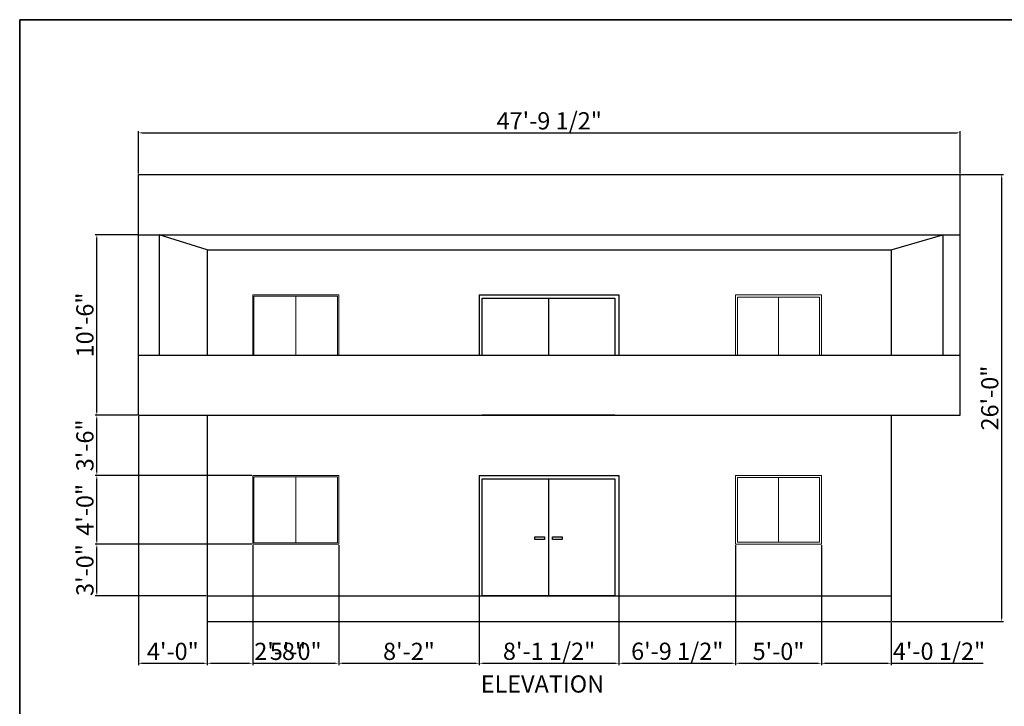
# Model space of a CAD drawing. Units: inches. Extents: x 2142 to 3604, y 1690 to 2981.
# Tile 4 of 9: x 2142 to 2829, y 2502 to 2981. Entities that reach past the tile are written whole.
import ezdxf

# ---------------------------------------------------------------- set-up
doc = ezdxf.new("R2010")
doc.units = ezdxf.units.IN
for name, color, linetype, lineweight in [('A-ANNO-DIMS', 2, 'Continuous', 18), ('A-ANNO-TEXT', 7, 'Continuous', 18), ('A-ANNO-TTLB', 7, 'Continuous', 35), ('A-DOOR', 4, 'Continuous', 25), ('A-ELEV', 7, 'Continuous', 25), ('A-GLAZ', 4, 'Continuous', 18)]:
    doc.layers.add(name, color=color, linetype=linetype, lineweight=lineweight)
doc.styles.get("Standard").update_dxf_attribs({"font": 'arial.ttf'})
doc.dimstyles.new('ISO-25', dxfattribs={"dimtxt": 12, "dimasz": 2.5, "dimexe": 1.25, "dimexo": 0.625, "dimtad": 1, "dimdec": 0, "dimlunit": 3, "dimtxsty": 'Standard', "dimcen": 2.5, "dimadec": 0, "dimazin": 0, "dimtfac": 1, "dimtdec": 0, "dimtmove": 0, "dimatfit": 3, "dimfxl": 1, "dimarcsym": 0})

# ---------------------------------------------------------------- blocks, each defined once
blk = doc.blocks.new('*D79')
at = {"layer": 'A-ANNO-DIMS', "color": 0, "lineweight": -2, "transparency": 16777216}
for p, q in [((2224.99, 2873.64), (2224.99, 2903.32)), ((2227.49, 2902.07), (2795.99, 2902.07)), ((2798.49, 2873.64), (2798.49, 2903.32))]:
    blk.add_line(p, q, dxfattribs=at)
at = {"layer": 'A-ANNO-DIMS', "color": 0, "transparency": 16777216}
for points in [[(2227.49, 2902.48), (2227.49, 2901.65), (2224.99, 2902.07)], [(2795.99, 2902.48), (2795.99, 2901.65), (2798.49, 2902.07)]]:
    blk.add_solid(points, dxfattribs=at)
at = {"layer": 'Defpoints', "color": 0, "transparency": 16777216}
for p in [(2798.49, 2902.07), (2224.99, 2873.02), (2798.49, 2873.02)]:
    blk.add_point(p, dxfattribs=at)
at = {"layer": 'A-ANNO-DIMS', "color": 0, "transparency": 16777216, "insert": (2511.74, 2908.9), "char_height": 12, "attachment_point": 5}
blk.add_mtext('47\'-9 1/2"', dxfattribs=at)
blk = doc.blocks.new('*D80')
at = {"layer": 'A-ANNO-DIMS', "color": 0, "lineweight": -2, "transparency": 16777216}
for p, q in [((2799.11, 2873.02), (2828.79, 2873.02)), ((2827.54, 2563.52), (2827.54, 2870.52)), ((2751.11, 2561.02), (2828.79, 2561.02))]:
    blk.add_line(p, q, dxfattribs=at)
at = {"layer": 'A-ANNO-DIMS', "color": 0, "transparency": 16777216}
for points in [[(2827.12, 2870.52), (2827.95, 2870.52), (2827.54, 2873.02)], [(2827.12, 2563.52), (2827.95, 2563.52), (2827.54, 2561.02)]]:
    blk.add_solid(points, dxfattribs=at)
at = {"layer": 'Defpoints', "color": 0, "transparency": 16777216}
for p in [(2798.49, 2873.02), (2827.54, 2873.02), (2750.49, 2561.02)]:
    blk.add_point(p, dxfattribs=at)
at = {"layer": 'A-ANNO-DIMS', "color": 0, "transparency": 16777216, "insert": (2820.78, 2717.02), "char_height": 12, "attachment_point": 5, "rotation": 90}
blk.add_mtext('26\'-0"', dxfattribs=at)
blk = doc.blocks.new('*D81')
at = {"layer": 'A-ANNO-DIMS', "color": 0, "lineweight": -2, "transparency": 16777216}
for p, q in [((2224.36, 2831.02), (2194.69, 2831.02)), ((2195.94, 2707.52), (2195.94, 2828.52)), ((2224.36, 2705.02), (2194.69, 2705.02))]:
    blk.add_line(p, q, dxfattribs=at)
at = {"layer": 'A-ANNO-DIMS', "color": 0, "transparency": 16777216}
for points in [[(2195.52, 2828.52), (2196.35, 2828.52), (2195.94, 2831.02)], [(2195.52, 2707.52), (2196.35, 2707.52), (2195.94, 2705.02)]]:
    blk.add_solid(points, dxfattribs=at)
at = {"layer": 'Defpoints', "color": 0, "transparency": 16777216}
for p in [(2195.94, 2831.02), (2224.99, 2831.02), (2224.99, 2705.02)]:
    blk.add_point(p, dxfattribs=at)
at = {"layer": 'A-ANNO-DIMS', "color": 0, "transparency": 16777216, "insert": (2189.18, 2768.02), "char_height": 12, "attachment_point": 5, "rotation": 90}
blk.add_mtext('10\'-6"', dxfattribs=at)
blk = doc.blocks.new('*D82')
at = {"layer": 'A-ANNO-DIMS', "color": 0, "lineweight": -2, "transparency": 16777216}
for p, q in [((2304.13, 2615.02), (2194.69, 2615.02)), ((2195.94, 2581.52), (2195.94, 2612.52)), ((2272.36, 2579.02), (2194.69, 2579.02))]:
    blk.add_line(p, q, dxfattribs=at)
at = {"layer": 'A-ANNO-DIMS', "color": 0, "transparency": 16777216}
for points in [[(2195.52, 2612.52), (2196.35, 2612.52), (2195.94, 2615.02)], [(2195.52, 2581.52), (2196.35, 2581.52), (2195.94, 2579.02)]]:
    blk.add_solid(points, dxfattribs=at)
at = {"layer": 'Defpoints', "color": 0, "transparency": 16777216}
for p in [(2195.94, 2615.02), (2304.76, 2615.02), (2272.99, 2579.02)]:
    blk.add_point(p, dxfattribs=at)
at = {"layer": 'A-ANNO-DIMS', "color": 0, "transparency": 16777216, "insert": (2189.18, 2597.02), "char_height": 12, "attachment_point": 5, "rotation": 90}
blk.add_mtext('3\'-0"', dxfattribs=at)
blk = doc.blocks.new('*D83')
at = {"layer": 'A-ANNO-DIMS', "color": 0, "lineweight": -2, "transparency": 16777216}
for p, q in [((2304.13, 2663.02), (2194.69, 2663.02)), ((2195.94, 2617.52), (2195.94, 2660.52)), ((2304.13, 2615.02), (2194.69, 2615.02))]:
    blk.add_line(p, q, dxfattribs=at)
at = {"layer": 'A-ANNO-DIMS', "color": 0, "transparency": 16777216}
for points in [[(2195.52, 2660.52), (2196.35, 2660.52), (2195.94, 2663.02)], [(2195.52, 2617.52), (2196.35, 2617.52), (2195.94, 2615.02)]]:
    blk.add_solid(points, dxfattribs=at)
at = {"layer": 'Defpoints', "color": 0, "transparency": 16777216}
for p in [(2195.94, 2663.02), (2304.76, 2663.02), (2304.76, 2615.02)]:
    blk.add_point(p, dxfattribs=at)
at = {"layer": 'A-ANNO-DIMS', "color": 0, "transparency": 16777216, "insert": (2189.18, 2639.02), "char_height": 12, "attachment_point": 5, "rotation": 90}
blk.add_mtext('4\'-0"', dxfattribs=at)
blk = doc.blocks.new('*D84')
at = {"layer": 'A-ANNO-DIMS', "color": 0, "lineweight": -2, "transparency": 16777216}
for p, q in [((2224.36, 2705.02), (2194.69, 2705.02)), ((2195.94, 2665.52), (2195.94, 2702.52)), ((2304.13, 2663.02), (2194.69, 2663.02))]:
    blk.add_line(p, q, dxfattribs=at)
at = {"layer": 'A-ANNO-DIMS', "color": 0, "transparency": 16777216}
for points in [[(2195.52, 2702.52), (2196.35, 2702.52), (2195.94, 2705.02)], [(2195.52, 2665.52), (2196.35, 2665.52), (2195.94, 2663.02)]]:
    blk.add_solid(points, dxfattribs=at)
at = {"layer": 'Defpoints', "color": 0, "transparency": 16777216}
for p in [(2195.94, 2705.02), (2224.99, 2705.02), (2304.76, 2663.02)]:
    blk.add_point(p, dxfattribs=at)
at = {"layer": 'A-ANNO-DIMS', "color": 0, "transparency": 16777216, "insert": (2189.18, 2684.02), "char_height": 12, "attachment_point": 5, "rotation": 90}
blk.add_mtext('3\'-6"', dxfattribs=at)
blk = doc.blocks.new('*D85')
at = {"layer": 'A-ANNO-DIMS', "color": 0, "lineweight": -2, "transparency": 16777216}
for p, q in [((2304.76, 2614.39), (2304.76, 2530.72)), ((2272.99, 2560.39), (2272.99, 2530.72)), ((2275.49, 2531.97), (2302.26, 2531.97)), ((2304.76, 2531.97), (2340.61, 2531.97))]:
    blk.add_line(p, q, dxfattribs=at)
at = {"layer": 'A-ANNO-DIMS', "color": 0, "transparency": 16777216}
for points in [[(2275.49, 2532.38), (2275.49, 2531.55), (2272.99, 2531.97)], [(2302.26, 2532.38), (2302.26, 2531.55), (2304.76, 2531.97)]]:
    blk.add_solid(points, dxfattribs=at)
at = {"layer": 'Defpoints', "color": 0, "transparency": 16777216}
for p in [(2304.76, 2615.02), (2272.99, 2561.02), (2304.76, 2531.97)]:
    blk.add_point(p, dxfattribs=at)
at = {"layer": 'A-ANNO-DIMS', "color": 0, "transparency": 16777216, "insert": (2323.93, 2538.72), "char_height": 12, "attachment_point": 5}
blk.add_mtext('2\'-8"', dxfattribs=at)
blk = doc.blocks.new('*D86')
at = {"layer": 'A-ANNO-DIMS', "color": 0, "lineweight": -2, "transparency": 16777216}
for p, q in [((2304.76, 2614.39), (2304.76, 2530.72)), ((2364.76, 2614.39), (2364.76, 2530.72)), ((2307.26, 2531.97), (2362.26, 2531.97))]:
    blk.add_line(p, q, dxfattribs=at)
at = {"layer": 'A-ANNO-DIMS', "color": 0, "transparency": 16777216}
for points in [[(2307.26, 2532.38), (2307.26, 2531.55), (2304.76, 2531.97)], [(2362.26, 2532.38), (2362.26, 2531.55), (2364.76, 2531.97)]]:
    blk.add_solid(points, dxfattribs=at)
at = {"layer": 'Defpoints', "color": 0, "transparency": 16777216}
for p in [(2304.76, 2615.02), (2364.76, 2615.02), (2364.76, 2531.97)]:
    blk.add_point(p, dxfattribs=at)
at = {"layer": 'A-ANNO-DIMS', "color": 0, "transparency": 16777216, "insert": (2334.76, 2538.72), "char_height": 12, "attachment_point": 5}
blk.add_mtext('5\'-0"', dxfattribs=at)
blk = doc.blocks.new('*D87')
at = {"layer": 'A-ANNO-DIMS', "color": 0, "lineweight": -2, "transparency": 16777216}
for p, q in [((2364.76, 2614.39), (2364.76, 2530.72)), ((2462.85, 2578.39), (2462.85, 2530.72)), ((2367.26, 2531.97), (2460.35, 2531.97))]:
    blk.add_line(p, q, dxfattribs=at)
at = {"layer": 'A-ANNO-DIMS', "color": 0, "transparency": 16777216}
for points in [[(2367.26, 2532.38), (2367.26, 2531.55), (2364.76, 2531.97)], [(2460.35, 2532.38), (2460.35, 2531.55), (2462.85, 2531.97)]]:
    blk.add_solid(points, dxfattribs=at)
at = {"layer": 'Defpoints', "color": 0, "transparency": 16777216}
for p in [(2364.76, 2615.02), (2462.85, 2579.02), (2462.85, 2531.97)]:
    blk.add_point(p, dxfattribs=at)
at = {"layer": 'A-ANNO-DIMS', "color": 0, "transparency": 16777216, "insert": (2413.81, 2538.72), "char_height": 12, "attachment_point": 5}
blk.add_mtext('8\'-2"', dxfattribs=at)
blk = doc.blocks.new('*D88')
at = {"layer": 'A-ANNO-DIMS', "color": 0, "lineweight": -2, "transparency": 16777216}
for p, q in [((2462.85, 2578.39), (2462.85, 2530.72)), ((2560.4, 2578.39), (2560.4, 2530.72)), ((2465.35, 2531.97), (2557.9, 2531.97))]:
    blk.add_line(p, q, dxfattribs=at)
at = {"layer": 'A-ANNO-DIMS', "color": 0, "transparency": 16777216}
for points in [[(2465.35, 2532.38), (2465.35, 2531.55), (2462.85, 2531.97)], [(2557.9, 2532.38), (2557.9, 2531.55), (2560.4, 2531.97)]]:
    blk.add_solid(points, dxfattribs=at)
at = {"layer": 'Defpoints', "color": 0, "transparency": 16777216}
for p in [(2462.85, 2579.02), (2560.4, 2579.02), (2560.4, 2531.97)]:
    blk.add_point(p, dxfattribs=at)
at = {"layer": 'A-ANNO-DIMS', "color": 0, "transparency": 16777216, "insert": (2511.63, 2538.8), "char_height": 12, "attachment_point": 5}
blk.add_mtext('8\'-1 1/2"', dxfattribs=at)
blk = doc.blocks.new('*D89')
at = {"layer": 'A-ANNO-DIMS', "color": 0, "lineweight": -2, "transparency": 16777216}
for p, q in [((2641.76, 2614.39), (2641.76, 2530.72)), ((2560.4, 2578.39), (2560.4, 2530.72)), ((2562.9, 2531.97), (2639.26, 2531.97))]:
    blk.add_line(p, q, dxfattribs=at)
at = {"layer": 'A-ANNO-DIMS', "color": 0, "transparency": 16777216}
for points in [[(2562.9, 2532.38), (2562.9, 2531.55), (2560.4, 2531.97)], [(2639.26, 2532.38), (2639.26, 2531.55), (2641.76, 2531.97)]]:
    blk.add_solid(points, dxfattribs=at)
at = {"layer": 'Defpoints', "color": 0, "transparency": 16777216}
for p in [(2641.76, 2615.02), (2560.4, 2579.02), (2641.76, 2531.97)]:
    blk.add_point(p, dxfattribs=at)
at = {"layer": 'A-ANNO-DIMS', "color": 0, "transparency": 16777216, "insert": (2601.08, 2538.8), "char_height": 12, "attachment_point": 5}
blk.add_mtext('6\'-9 1/2"', dxfattribs=at)
blk = doc.blocks.new('*D90')
at = {"layer": 'A-ANNO-DIMS', "color": 0, "lineweight": -2, "transparency": 16777216}
for p, q in [((2641.76, 2614.39), (2641.76, 2530.72)), ((2701.76, 2614.39), (2701.76, 2530.72)), ((2644.26, 2531.97), (2699.26, 2531.97))]:
    blk.add_line(p, q, dxfattribs=at)
at = {"layer": 'A-ANNO-DIMS', "color": 0, "transparency": 16777216}
for points in [[(2644.26, 2532.38), (2644.26, 2531.55), (2641.76, 2531.97)], [(2699.26, 2532.38), (2699.26, 2531.55), (2701.76, 2531.97)]]:
    blk.add_solid(points, dxfattribs=at)
at = {"layer": 'Defpoints', "color": 0, "transparency": 16777216}
for p in [(2641.76, 2615.02), (2701.76, 2615.02), (2701.76, 2531.97)]:
    blk.add_point(p, dxfattribs=at)
at = {"layer": 'A-ANNO-DIMS', "color": 0, "transparency": 16777216, "insert": (2671.76, 2538.72), "char_height": 12, "attachment_point": 5}
blk.add_mtext('5\'-0"', dxfattribs=at)
blk = doc.blocks.new('*D91')
at = {"layer": 'A-ANNO-DIMS', "color": 0, "lineweight": -2, "transparency": 16777216}
for p, q in [((2701.76, 2614.39), (2701.76, 2530.72)), ((2750.49, 2560.39), (2750.49, 2530.72)), ((2704.26, 2531.97), (2747.99, 2531.97)), ((2750.49, 2531.97), (2814.58, 2531.97))]:
    blk.add_line(p, q, dxfattribs=at)
at = {"layer": 'A-ANNO-DIMS', "color": 0, "transparency": 16777216}
for points in [[(2704.26, 2532.38), (2704.26, 2531.55), (2701.76, 2531.97)], [(2747.99, 2532.38), (2747.99, 2531.55), (2750.49, 2531.97)]]:
    blk.add_solid(points, dxfattribs=at)
at = {"layer": 'Defpoints', "color": 0, "transparency": 16777216}
for p in [(2701.76, 2615.02), (2750.49, 2561.02), (2750.49, 2531.97)]:
    blk.add_point(p, dxfattribs=at)
at = {"layer": 'A-ANNO-DIMS', "color": 0, "transparency": 16777216, "insert": (2783.78, 2538.8), "char_height": 12, "attachment_point": 5}
blk.add_mtext('4\'-0 1/2"', dxfattribs=at)
blk = doc.blocks.new('*D92')
at = {"layer": 'A-ANNO-DIMS', "color": 0, "lineweight": -2, "transparency": 16777216}
for p, q in [((2224.99, 2704.39), (2224.99, 2530.72)), ((2272.99, 2704.39), (2272.99, 2530.72)), ((2227.49, 2531.97), (2270.49, 2531.97))]:
    blk.add_line(p, q, dxfattribs=at)
at = {"layer": 'A-ANNO-DIMS', "color": 0, "transparency": 16777216}
for points in [[(2227.49, 2532.38), (2227.49, 2531.55), (2224.99, 2531.97)], [(2270.49, 2532.38), (2270.49, 2531.55), (2272.99, 2531.97)]]:
    blk.add_solid(points, dxfattribs=at)
at = {"layer": 'Defpoints', "color": 0, "transparency": 16777216}
for p in [(2224.99, 2705.02), (2272.99, 2705.02), (2272.99, 2531.97)]:
    blk.add_point(p, dxfattribs=at)
at = {"layer": 'A-ANNO-DIMS', "color": 0, "transparency": 16777216, "insert": (2248.99, 2538.72), "char_height": 12, "attachment_point": 5}
blk.add_mtext('4\'-0"', dxfattribs=at)

msp = doc.modelspace()

# ---------------------------------------------------------------- linework, layer by layer
at = {"layer": 'A-ANNO-TTLB'}
msp.add_lwpolyline([(2142.1, 2981.01), (3604.42, 2981.01), (3604.42, 1690.13), (2142.1, 1690.13)], close=True, dxfattribs=at)
at = {"layer": 'A-DOOR'}
for p, q in [((2462.85, 2789.02), (2462.85, 2747.02)), ((2462.85, 2789.02), (2560.4, 2789.02)), ((2511.25, 2786.76), (2511.25, 2747.02)), ((2560.4, 2789.02), (2560.4, 2747.02)), ((2462.85, 2663.02), (2462.85, 2579.02)), ((2462.85, 2663.02), (2560.4, 2663.02)), ((2511.25, 2660.76), (2511.25, 2579.02)), ((2560.4, 2663.02), (2560.4, 2579.02))]:
    msp.add_line(p, q, dxfattribs=at)
for points in [[(2464.91, 2747.02), (2464.91, 2786.76), (2557.59, 2786.76), (2557.59, 2747.02)], [(2557.59, 2705.02), (2557.59, 2705.02), (2464.91, 2705.02)]]:
    msp.add_lwpolyline(points, dxfattribs=at)
for points in [[(2464.91, 2660.76), (2557.59, 2660.76), (2557.59, 2579.02), (2464.91, 2579.02)], [(2501.67, 2620.16), (2508.36, 2620.16), (2508.36, 2618.29), (2501.67, 2618.29)], [(2513.99, 2620.16), (2520.68, 2620.16), (2520.68, 2618.29), (2513.99, 2618.29)]]:
    msp.add_lwpolyline(points, close=True, dxfattribs=at)
at = {"layer": 'A-ELEV'}
for p, q in [((2224.99, 2873.02), (2798.49, 2873.02)), ((2224.99, 2705.02), (2224.99, 2873.02)), ((2798.49, 2705.02), (2798.49, 2873.02)), ((2224.99, 2831.02), (2798.49, 2831.02)), ((2239.52, 2831.02), (2239.52, 2747.02)), ((2272.99, 2820.43), (2239.52, 2831.02)), ((2750.49, 2820.43), (2786.39, 2831.02)), ((2786.39, 2831.02), (2786.39, 2747.02)), ((2272.99, 2820.43), (2272.99, 2747.02)), ((2272.99, 2820.43), (2750.49, 2820.43)), ((2750.49, 2820.43), (2750.49, 2747.02)), ((2224.99, 2747.02), (2798.49, 2747.02)), ((2224.99, 2705.02), (2798.49, 2705.02)), ((2272.99, 2705.02), (2272.99, 2561.02)), ((2272.99, 2705.02), (2272.99, 2687.02)), ((2750.49, 2705.02), (2750.49, 2561.02)), ((2750.49, 2705.02), (2750.49, 2687.02)), ((2272.99, 2579.02), (2750.49, 2579.02)), ((2272.99, 2561.02), (2750.49, 2561.02))]:
    msp.add_line(p, q, dxfattribs=at)
at = {"layer": 'A-GLAZ'}
for p, q in [((2304.76, 2789.02), (2304.76, 2747.02)), ((2304.76, 2789.02), (2364.76, 2789.02)), ((2334.74, 2788.03), (2334.74, 2747.02)), ((2364.76, 2789.02), (2364.76, 2747.02)), ((2641.76, 2789.02), (2641.76, 2747.02)), ((2641.76, 2789.02), (2701.76, 2789.02)), ((2671.73, 2787.51), (2671.73, 2747.02)), ((2701.76, 2789.02), (2701.76, 2747.02)), ((2304.76, 2663.02), (2304.76, 2615.02)), ((2304.76, 2663.02), (2364.76, 2663.02)), ((2334.74, 2662.03), (2334.74, 2615.89)), ((2364.76, 2663.02), (2364.76, 2615.02)), ((2641.76, 2663.02), (2641.76, 2615.02)), ((2641.76, 2663.02), (2701.76, 2663.02)), ((2671.73, 2661.51), (2671.73, 2616.56)), ((2701.76, 2663.02), (2701.76, 2615.02)), ((2304.76, 2615.02), (2364.76, 2615.02)), ((2641.76, 2615.02), (2701.76, 2615.02))]:
    msp.add_line(p, q, dxfattribs=at)
for points in [[(2305.55, 2747.02), (2305.55, 2788.03), (2363.94, 2788.03), (2363.94, 2747.02)], [(2643.09, 2747.02), (2643.09, 2787.51), (2700.37, 2787.51), (2700.37, 2747.02)]]:
    msp.add_lwpolyline(points, dxfattribs=at)
for points in [[(2305.55, 2662.03), (2363.94, 2662.03), (2363.94, 2615.89), (2305.55, 2615.89)], [(2643.09, 2661.51), (2700.37, 2661.51), (2700.37, 2616.56), (2643.09, 2616.56)]]:
    msp.add_lwpolyline(points, close=True, dxfattribs=at)

# ---------------------------------------------------------------- texts
at = {"layer": 'A-ANNO-TEXT', "insert": (2463.89, 2523.52), "char_height": 12, "attachment_point": 1}
msp.add_mtext_dynamic_manual_height_columns('ELEVATION', width=336.8938, gutter_width=12.5, heights=[0], dxfattribs=at)

# ---------------------------------------------------------------- dimensions: what is measured, and where the dimension line sits
at = {"layer": 'A-ANNO-DIMS'}
for base, p1, p2, picture, middle in [((2798.49, 2902.07), (2224.99, 2873.02), (2798.49, 2873.02), '*D79', (2511.74, 2908.9)), ((2272.99, 2531.97), (2224.99, 2705.02), (2272.99, 2705.02), '*D92', (2248.99, 2538.72)), ((2304.76, 2531.97), (2272.99, 2561.02), (2304.76, 2615.02), '*D85', (2323.93, 2538.72)), ((2364.76, 2531.97), (2304.76, 2615.02), (2364.76, 2615.02), '*D86', (2334.76, 2538.72)), ((2462.85, 2531.97), (2364.76, 2615.02), (2462.85, 2579.02), '*D87', (2413.81, 2538.72)), ((2641.76, 2531.97), (2560.4, 2579.02), (2641.76, 2615.02), '*D89', (2601.08, 2538.8)), ((2701.76, 2531.97), (2641.76, 2615.02), (2701.76, 2615.02), '*D90', (2671.76, 2538.72)), ((2750.49, 2531.97), (2701.76, 2615.02), (2750.49, 2561.02), '*D91', (2783.78, 2538.8)), ((2560.4008, 2531.9672), (2462.8534, 2579.0172), (2560.4008, 2579.0172), '*D88', (2511.6271, 2538.7969))]:
    dim = msp.add_linear_dim(base=base, p1=p1, p2=p2, dimstyle='ISO-25', override={"dimdec": 1, "dimlfac": 1, "dimrnd": 0, "dimzin": 1, "dimdsep": 46, "dimlunit": 4, "dimfrac": 2}, dxfattribs=at)
    dim.commit()
    dim.dimension.update_dxf_attribs({"geometry": picture, "text_midpoint": middle})
for base, p1, p2, picture, middle in [((2827.54, 2873.02), (2750.49, 2561.02), (2798.49, 2873.02), '*D80', (2820.78, 2717.02)), ((2195.94, 2831.02), (2224.99, 2705.02), (2224.99, 2831.02), '*D81', (2189.18, 2768.02)), ((2195.94, 2705.02), (2304.76, 2663.02), (2224.99, 2705.02), '*D84', (2189.18, 2684.02)), ((2195.94, 2663.02), (2304.76, 2615.02), (2304.76, 2663.02), '*D83', (2189.18, 2639.02)), ((2195.94, 2615.02), (2272.99, 2579.02), (2304.76, 2615.02), '*D82', (2189.18, 2597.02))]:
    dim = msp.add_linear_dim(base=base, p1=p1, p2=p2, angle=90, dimstyle='ISO-25', override={"dimdec": 1, "dimlfac": 1, "dimrnd": 0, "dimzin": 1, "dimdsep": 46, "dimlunit": 4, "dimfrac": 2}, dxfattribs=at)
    dim.commit()
    dim.dimension.update_dxf_attribs({"geometry": picture, "text_midpoint": middle})

doc.saveas('drawing.dxf')
